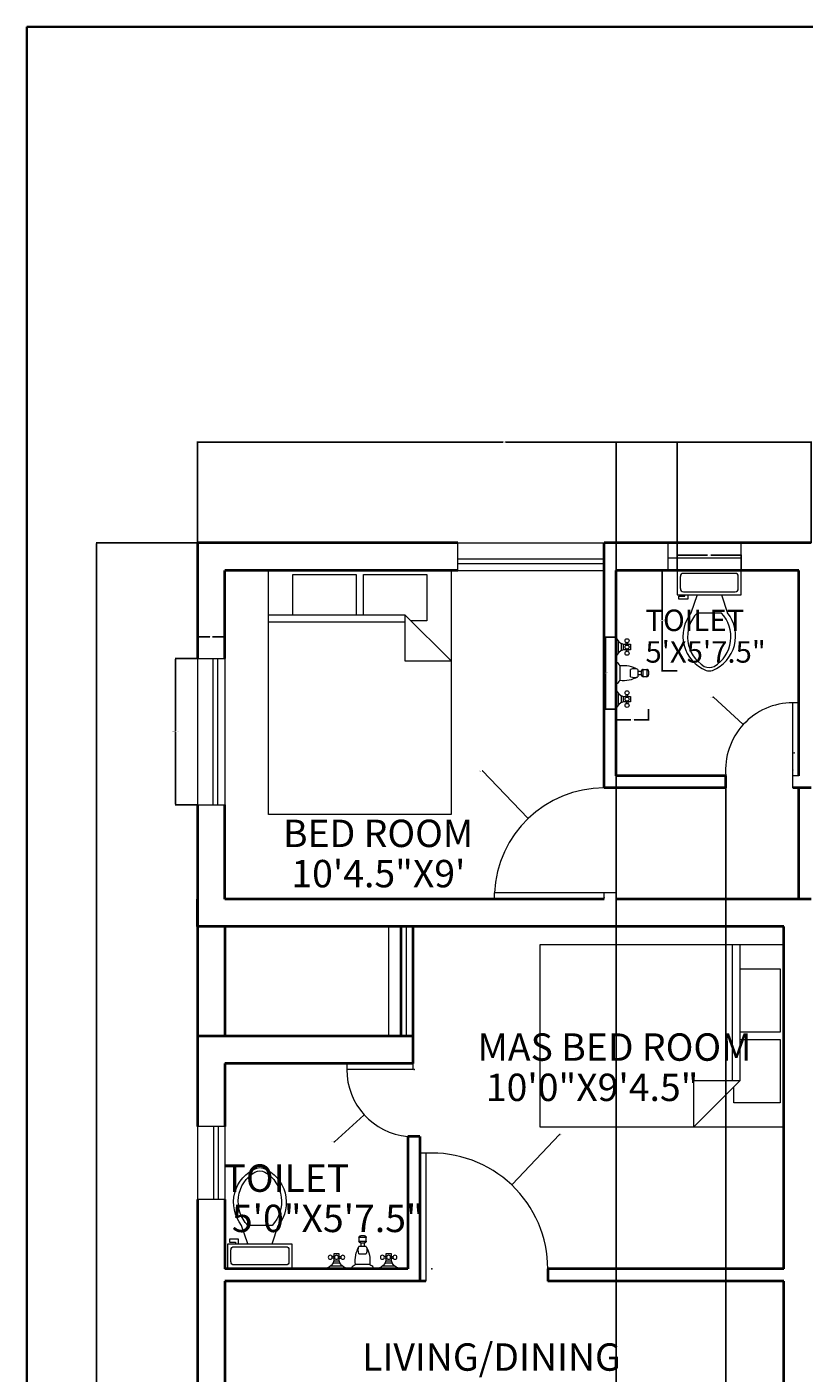
# Model space of a CAD drawing. Units: inches. Extents: x 2220 to 3422, y 783 to 1748.
# Tile 4 of 7: x 2220 to 2475, y 1306 to 1748. Entities that reach past the tile are written whole.
import ezdxf

# ---------------------------------------------------------------- set-up
doc = ezdxf.new("R2010")
doc.units = ezdxf.units.IN
for name, color, linetype, lineweight in [('A-ANNO-DIMS', 2, 'Continuous', 18), ('A-ANNO-TTLB', 7, 'Continuous', 35), ('A-AREA-IDEN', 7, 'Continuous', 18), ('A-DOOR', 3, 'Continuous', 20), ('A-FLOR-FIXT', 9, 'Continuous', 18), ('A-FURN', 8, 'Continuous', 18), ('A-GLAZ', 4, 'Continuous', 18), ('A-WALL', 7, 'Continuous', 40)]:
    doc.layers.add(name, color=color, linetype=linetype, lineweight=lineweight)
doc.styles.get("Standard").update_dxf_attribs({"font": 'arial.ttf'})
doc.dimstyles.get("Standard").update_dxf_attribs({"dimtxt": 0.18, "dimasz": 0.18, "dimexe": 0.18, "dimexo": 0.0625, "dimgap": 0.09, "dimtad": 0, "dimtih": 1, "dimtoh": 1, "dimdec": 4, "dimzin": 0, "dimdsep": 46, "dimtxsty": 'Standard', "dimcen": 0.09, "dimadec": 0, "dimazin": 0, "dimtfac": 1, "dimtdec": 4, "dimtofl": 0, "dimtmove": 0, "dimatfit": 3, "dimfxl": 1, "dimtolj": 1, "dimtzin": 0, "dimarcsym": 0})

# ---------------------------------------------------------------- blocks, each defined once
blk = doc.blocks.new('Toilet - top')
for p, q in [((9.5, -6), (9.5, -2)), ((-10, -8.5), (-8, -8.5)), ((-10, -9.5), (-10, -8.5)), ((-8, -8.5), (-8, -8)), ((-7, -8), (-7, -9.5)), ((-4, -8), (-6, -14)), ((4, -8), (6, -14)), ((-7, -9.5), (-10, -9.5)), ((4, -14), (-4, -14))]:
    blk.add_line(p, q)
blk.add_lwpolyline([(10.5, -8), (10.5, 0), (-10.5, 0), (-10.5, -8)], close=True)
for points in [[(-9.5, -2), (-9.5, -6)], [(8.5, -1), (-8.5, -1)], [(-8.5, -7), (8.5, -7)]]:
    blk.add_lwpolyline(points)
for centre, radius, start, end in [((-8.62, -1.88), 0.884, 81.8699, 188.1301), ((8.62, -1.88), 0.884, 351.8699, 98.1301), ((-8.62, -6.12), 0.884, 171.8699, 278.1301), ((8.62, -6.12), 0.884, 261.8699, 8.1301), ((3.52, -21.58), 12.17, 141.4691, 247.9714), ((4.2, -21.82), 11.33, 136.3677, 238.9468), ((-3.52, -21.58), 12.17, 292.0284, 38.5307), ((-4.2, -21.82), 11.33, 301.053, 43.6321), ((0, -27.88), 4, 245.7318, 294.2682), ((0, -29), 4, 254.8605, 285.1395)]:
    blk.add_arc(centre, radius, start, end)
blk = doc.blocks.new('Faucet - Bathroom front')
for p, q in [((-0.5, 4.25), (0.5, 4.25)), ((0.5, 3.75), (-0.5, 3.75)), ((-0.5, 3), (0.5, 3)), ((0.5, 2), (-0.5, 2)), ((-0.25, 3), (-0.25, 3.5)), ((0.25, 3.5), (0.25, 3)), ((-5, 0), (-2.25, 0)), ((-4.5087, 0.25), (-2.7408, 0.25)), ((-4, 1.625), (-4.25, 1.625)), ((-4, 1.375), (-4.25, 1.375)), ((-3.1442, 0.75), (-4.0979, 0.75)), ((-3.25, 1.625), (-3, 1.625)), ((-3.25, 1.375), (-3, 1.375)), ((-1.5, 0), (1.5, 0)), ((-1, 0.5), (1, 0.5)), ((2.25, 0), (5, 0)), ((2.7413, 0.25), (4.5092, 0.25)), ((3.25, 1.625), (3, 1.625)), ((3.25, 1.375), (3, 1.375)), ((4.1058, 0.75), (3.1521, 0.75)), ((4, 1.625), (4.25, 1.625)), ((4, 1.375), (4.25, 1.375))]:
    blk.add_line(p, q)
for points in [[(-0.5, 3.75), (-0.5, 4.25)], [(-0.25, 4.5), (0.25, 4.5)], [(0.5, 4.25), (0.5, 3.75)], [(0.25, 3.5), (-0.25, 3.5)]]:
    blk.add_lwpolyline(points)
for points in [[(-4, 1), (-4, 2), (-3.25, 2), (-3.25, 1)], [(3.25, 1), (3.25, 2), (4, 2), (4, 1)]]:
    blk.add_lwpolyline(points, close=True)
for centre in [(-4.5, 1.5), (-3.625, 1.5), (-2.75, 1.5), (2.75, 1.5), (3.625, 1.5), (4.5, 1.5)]:
    blk.add_circle(centre, 0.2795)
for centre, radius, start, end in [((-0.2575, 4.2575), 0.2426, 88.22243, 181.7776), ((-0.2575, 3.7425), 0.2426, 178.2224, 271.7776), ((0.2575, 4.2575), 0.2426, 358.2224, 91.77757), ((0.2575, 3.7425), 0.2426, 268.2224, 1.777565), ((3, 1), 4.0311, 150.2551, 187.125), ((0.6413, 2.5), 1.246, 156.3417, 203.6583), ((-3, 1), 4.0311, 352.875, 29.74488), ((-0.6413, 2.5), 1.246, 336.3417, 23.65835), ((-5.375, 1.375), 1.4252, 285.2551, 344.7449), ((-1.875, 1.375), 1.4252, 195.2551, 254.7449), ((-0.7962, -0.2038), 0.7327, 106.1502, 163.8498), ((0.7962, -0.2038), 0.7327, 16.1502, 73.84979), ((1.875, 1.375), 1.4252, 285.2551, 344.7449), ((5.375, 1.375), 1.4252, 195.2551, 254.7449)]:
    blk.add_arc(centre, radius, start, end)
blk = doc.blocks.new('Bed - Queen')
for p, q in [((0, -80.00003), (0, 0)), ((0, 0), (59.99999, 0)), ((59.99999, 0), (59.99999, -80.00003)), ((7.99999, -1.2), (28.79998, -1.2)), ((7.99999, -14.4), (7.99999, -1.2)), ((28.79998, -1.2), (28.79998, -14.4)), ((31.19999, -1.2), (51.99999, -1.2)), ((31.19999, -14.4), (31.19999, -1.2)), ((51.99999, -1.2), (51.99999, -16.4)), ((0, -14.4), (44.8, -14.4)), ((44.8, -16.8), (0, -16.8)), ((59.99999, -29.6), (44.8, -14.4)), ((44.8, -14.4), (44.8, -29.6)), ((51.99999, -16.4), (46.79936, -16.4)), ((44.8, -29.6), (59.99999, -29.6)), ((59.99999, -80.00003), (0, -80.00003))]:
    blk.add_line(p, q)
blk = doc.blocks.new('WIN-48-OFFSET-B')
for p, q in [((0, 48), (9, 48)), ((0, 48), (0, 0)), ((5, 48), (5, 0)), ((6.5, 48), (6.5, 0)), ((9, 48), (9, 0)), ((0, 0), (9, 0))]:
    blk.add_line(p, q)
blk = doc.blocks.new('*D21')
at = {"layer": 'A-ANNO-DIMS', "color": 0, "lineweight": -2, "transparency": 16777216}
for p, q in [((2433.53, 1569.38), (2428.45, 1569.38)), ((2428.63, 1569.2), (2428.63, 1553.04)), ((2428.63, 1536.51), (2428.63, 1552.67)), ((2433.53, 1536.33), (2428.45, 1536.33))]:
    blk.add_line(p, q, dxfattribs=at)
at = {"layer": 'A-ANNO-DIMS', "color": 0, "transparency": 16777216}
for points in [[(2428.6, 1569.2), (2428.66, 1569.2), (2428.63, 1569.38)], [(2428.6, 1536.51), (2428.66, 1536.51), (2428.63, 1536.33)]]:
    blk.add_solid(points, dxfattribs=at)
at = {"layer": 'Defpoints', "color": 0, "transparency": 16777216}
for p in [(2428.63, 1569.38), (2433.59, 1569.38), (2433.59, 1536.33)]:
    blk.add_point(p, dxfattribs=at)
at = {"layer": 'A-ANNO-DIMS', "color": 0, "transparency": 16777216, "insert": (2428.63, 1552.86), "char_height": 0.18, "attachment_point": 5}
blk.add_mtext('\\A1;WC 33 TYP.', dxfattribs=at)
blk = doc.blocks.new('*D22')
at = {"layer": 'A-ANNO-DIMS', "color": 0, "lineweight": -2, "transparency": 16777216}
for p, q in [((2433.59, 1569.44), (2433.59, 1574.52)), ((2433.77, 1574.34), (2443.56, 1574.34)), ((2454.41, 1574.34), (2444.62, 1574.34)), ((2454.59, 1569.44), (2454.59, 1574.52))]:
    blk.add_line(p, q, dxfattribs=at)
at = {"layer": 'A-ANNO-DIMS', "color": 0, "transparency": 16777216}
for points in [[(2433.77, 1574.37), (2433.77, 1574.31), (2433.59, 1574.34)], [(2454.41, 1574.37), (2454.41, 1574.31), (2454.59, 1574.34)]]:
    blk.add_solid(points, dxfattribs=at)
at = {"layer": 'Defpoints', "color": 0, "transparency": 16777216}
for p in [(2454.59, 1574.34), (2433.59, 1569.38), (2454.59, 1569.38)]:
    blk.add_point(p, dxfattribs=at)
at = {"layer": 'A-ANNO-DIMS', "color": 0, "transparency": 16777216, "insert": (2444.09, 1574.34), "char_height": 0.18, "attachment_point": 5}
blk.add_mtext('\\A1;21 TYP.', dxfattribs=at)
blk = doc.blocks.new('*D23')
at = {"layer": 'A-ANNO-DIMS', "color": 0, "lineweight": -2, "transparency": 16777216}
for p, q in [((2413.48, 1547.45), (2409.82, 1547.45)), ((2410, 1547.27), (2410, 1535.82)), ((2410, 1524.01), (2410, 1535.46)), ((2413.48, 1523.83), (2409.82, 1523.83))]:
    blk.add_line(p, q, dxfattribs=at)
at = {"layer": 'A-ANNO-DIMS', "color": 0, "transparency": 16777216}
for points in [[(2409.97, 1547.27), (2410.03, 1547.27), (2410, 1547.45)], [(2409.97, 1524.01), (2410.03, 1524.01), (2410, 1523.83)]]:
    blk.add_solid(points, dxfattribs=at)
at = {"layer": 'Defpoints', "color": 0, "transparency": 16777216}
for p in [(2413.55, 1547.45), (2410, 1523.83), (2413.55, 1523.83)]:
    blk.add_point(p, dxfattribs=at)
at = {"layer": 'A-ANNO-DIMS', "color": 0, "transparency": 16777216, "insert": (2410, 1535.64), "char_height": 0.18, "attachment_point": 5}
blk.add_mtext('\\A1;LAV. TAP 24 TYP.', dxfattribs=at)
blk = doc.blocks.new('*D24')
at = {"layer": 'A-ANNO-DIMS', "color": 0, "lineweight": -2, "transparency": 16777216}
for p, q in [((2413.55, 1523.77), (2413.55, 1520.11)), ((2424.18, 1523.77), (2424.18, 1520.11)), ((2413.73, 1520.29), (2418.34, 1520.29)), ((2424, 1520.29), (2419.38, 1520.29))]:
    blk.add_line(p, q, dxfattribs=at)
at = {"layer": 'A-ANNO-DIMS', "color": 0, "transparency": 16777216}
for points in [[(2413.73, 1520.32), (2413.73, 1520.26), (2413.55, 1520.29)], [(2424, 1520.32), (2424, 1520.26), (2424.18, 1520.29)]]:
    blk.add_solid(points, dxfattribs=at)
at = {"layer": 'Defpoints', "color": 0, "transparency": 16777216}
for p in [(2413.55, 1523.83), (2424.18, 1523.83), (2424.18, 1520.29)]:
    blk.add_point(p, dxfattribs=at)
at = {"layer": 'A-ANNO-DIMS', "color": 0, "transparency": 16777216, "insert": (2418.86, 1520.29), "char_height": 0.18, "attachment_point": 5}
blk.add_mtext('\\A1;11 TYP.', dxfattribs=at)
blk = doc.blocks.new('*D49')
at = {"layer": 'A-ANNO-DIMS', "color": 0, "lineweight": -2, "transparency": 16777216}
for p, q in [((2275.98, 1540.39), (2268.67, 1540.39)), ((2268.85, 1540.21), (2268.85, 1516.57)), ((2268.85, 1492.57), (2268.85, 1516.21)), ((2275.98, 1492.39), (2268.67, 1492.39))]:
    blk.add_line(p, q, dxfattribs=at)
at = {"layer": 'A-ANNO-DIMS', "color": 0, "transparency": 16777216}
for points in [[(2268.82, 1540.21), (2268.88, 1540.21), (2268.85, 1540.39)], [(2268.82, 1492.57), (2268.88, 1492.57), (2268.85, 1492.39)]]:
    blk.add_solid(points, dxfattribs=at)
at = {"layer": 'Defpoints', "color": 0, "transparency": 16777216}
for p in [(2268.85, 1540.39), (2276.05, 1540.39), (2276.05, 1492.39)]:
    blk.add_point(p, dxfattribs=at)
at = {"layer": 'A-ANNO-DIMS', "color": 0, "transparency": 16777216, "insert": (2268.85, 1516.39), "char_height": 0.18, "attachment_point": 5}
blk.add_mtext('\\A1;WINDOW B 48 TYP.', dxfattribs=at)
blk = doc.blocks.new('*D50')
at = {"layer": 'A-ANNO-DIMS', "color": 0, "lineweight": -2, "transparency": 16777216}
for p, q in [((2276.05, 1540.45), (2276.05, 1547.77)), ((2276.23, 1547.59), (2280.09, 1547.59)), ((2284.87, 1547.59), (2281, 1547.59)), ((2285.05, 1540.45), (2285.05, 1547.77))]:
    blk.add_line(p, q, dxfattribs=at)
at = {"layer": 'A-ANNO-DIMS', "color": 0, "transparency": 16777216}
for points in [[(2276.23, 1547.62), (2276.23, 1547.56), (2276.05, 1547.59)], [(2284.87, 1547.62), (2284.87, 1547.56), (2285.05, 1547.59)]]:
    blk.add_solid(points, dxfattribs=at)
at = {"layer": 'Defpoints', "color": 0, "transparency": 16777216}
for p in [(2285.05, 1547.59), (2276.05, 1540.39), (2285.05, 1540.39)]:
    blk.add_point(p, dxfattribs=at)
at = {"layer": 'A-ANNO-DIMS', "color": 0, "transparency": 16777216, "insert": (2280.55, 1547.59), "char_height": 0.18, "attachment_point": 5}
blk.add_mtext('\\A1;9 TYP.', dxfattribs=at)
blk = doc.blocks.new('*D54')
at = {"layer": 'A-ANNO-DIMS', "color": 0, "lineweight": -2, "transparency": 16777216}
for p, q in [((2275.98, 1578.39), (2242.72, 1578.39)), ((2242.9, 1578.21), (2242.9, 1255.07)), ((2242.9, 931.57), (2242.9, 1254.71)), ((2275.98, 931.39), (2242.72, 931.39))]:
    blk.add_line(p, q, dxfattribs=at)
at = {"layer": 'A-ANNO-DIMS', "color": 0, "transparency": 16777216}
for points in [[(2242.87, 1578.21), (2242.93, 1578.21), (2242.9, 1578.39)], [(2242.87, 931.57), (2242.93, 931.57), (2242.9, 931.39)]]:
    blk.add_solid(points, dxfattribs=at)
at = {"layer": 'Defpoints', "color": 0, "transparency": 16777216}
for p in [(2242.9, 1578.39), (2276.05, 1578.39), (2276.05, 931.39)]:
    blk.add_point(p, dxfattribs=at)
at = {"layer": 'A-ANNO-DIMS', "color": 0, "transparency": 16777216, "insert": (2242.9, 1254.89), "char_height": 0.18, "attachment_point": 5}
blk.add_mtext('\\A1;647', dxfattribs=at)
blk = doc.blocks.new('*D58')
at = {"layer": 'A-ANNO-DIMS', "color": 0, "lineweight": -2, "transparency": 16777216}
for p, q in [((2276.05, 1578.45), (2276.05, 1611.72)), ((2276.23, 1611.54), (2376.4, 1611.54)), ((2477.37, 1611.54), (2377.19, 1611.54)), ((2477.55, 1578.45), (2477.55, 1611.72))]:
    blk.add_line(p, q, dxfattribs=at)
at = {"layer": 'A-ANNO-DIMS', "color": 0, "transparency": 16777216}
for points in [[(2276.23, 1611.57), (2276.23, 1611.51), (2276.05, 1611.54)], [(2477.37, 1611.57), (2477.37, 1611.51), (2477.55, 1611.54)]]:
    blk.add_solid(points, dxfattribs=at)
at = {"layer": 'Defpoints', "color": 0, "transparency": 16777216}
for p in [(2477.55, 1611.54), (2276.05, 1578.39), (2477.55, 1578.39)]:
    blk.add_point(p, dxfattribs=at)
at = {"layer": 'A-ANNO-DIMS', "color": 0, "transparency": 16777216, "insert": (2376.8, 1611.54), "char_height": 0.18, "attachment_point": 5}
blk.add_mtext('\\A1;201.5', dxfattribs=at)
blk = doc.blocks.new('*D72')
at = {"layer": 'A-ANNO-DIMS', "color": 0, "lineweight": -2, "transparency": 16777216}
for p, q in [((2413.55, 1569.45), (2413.55, 1611.72)), ((2413.73, 1611.54), (2423.1, 1611.54)), ((2433.41, 1611.54), (2424.04, 1611.54)), ((2433.59, 1569.44), (2433.59, 1611.72))]:
    blk.add_line(p, q, dxfattribs=at)
at = {"layer": 'A-ANNO-DIMS', "color": 0, "transparency": 16777216}
for points in [[(2413.73, 1611.57), (2413.73, 1611.51), (2413.55, 1611.54)], [(2433.41, 1611.57), (2433.41, 1611.51), (2433.59, 1611.54)]]:
    blk.add_solid(points, dxfattribs=at)
at = {"layer": 'Defpoints', "color": 0, "transparency": 16777216}
for p in [(2433.59, 1611.54), (2413.55, 1569.39), (2433.59, 1569.38)]:
    blk.add_point(p, dxfattribs=at)
at = {"layer": 'A-ANNO-DIMS', "color": 0, "transparency": 16777216, "insert": (2423.57, 1611.54), "char_height": 0.18, "attachment_point": 5}
blk.add_mtext('\\A1;20.045', dxfattribs=at)
blk = doc.blocks.new('*D73')
at = {"layer": 'A-ANNO-DIMS', "color": 0, "lineweight": -2, "transparency": 16777216}
for p, q in [((2413.55, 1501.83), (2413.55, 898.06)), ((2449.55, 1501.83), (2449.55, 898.06)), ((2413.73, 898.24), (2431.33, 898.24)), ((2449.37, 898.24), (2431.77, 898.24))]:
    blk.add_line(p, q, dxfattribs=at)
at = {"layer": 'A-ANNO-DIMS', "color": 0, "transparency": 16777216}
for points in [[(2413.73, 898.27), (2413.73, 898.21), (2413.55, 898.24)], [(2449.37, 898.27), (2449.37, 898.21), (2449.55, 898.24)]]:
    blk.add_solid(points, dxfattribs=at)
at = {"layer": 'Defpoints', "color": 0, "transparency": 16777216}
for p in [(2413.55, 1501.89), (2449.55, 1501.89), (2449.55, 898.24)]:
    blk.add_point(p, dxfattribs=at)
at = {"layer": 'A-ANNO-DIMS', "color": 0, "transparency": 16777216, "insert": (2431.55, 898.24), "char_height": 0.18, "attachment_point": 5}
blk.add_mtext('\\A1;36', dxfattribs=at)
blk = doc.blocks.new('*D78')
at = {"layer": 'A-ANNO-DIMS', "color": 0, "lineweight": -2, "transparency": 16777216}
for p, q in [((2394.93, 1384.03), (2379.33, 1367.61)), ((2395.11, 1384.03), (2394.93, 1384.03)), ((2352.91, 1339.89), (2353.09, 1339.89)), ((2353, 1339.8), (2353, 1339.98))]:
    blk.add_line(p, q, dxfattribs=at)
at = {"layer": 'A-ANNO-DIMS', "color": 0, "transparency": 16777216}
blk.add_solid([(2379.31, 1367.63), (2379.35, 1367.59), (2379.2, 1367.48)], dxfattribs=at)
at = {"layer": 'Defpoints', "color": 0, "transparency": 16777216}
for p in [(2379.2, 1367.48), (2353, 1339.89)]:
    blk.add_point(p, dxfattribs=at)
at = {"layer": 'A-ANNO-DIMS', "color": 0, "transparency": 16777216, "insert": (2395.59, 1384.03), "char_height": 0.18, "attachment_point": 5}
blk.add_mtext('\\A1;R38.05', dxfattribs=at)
blk = doc.blocks.new('*D79')
at = {"layer": 'A-ANNO-DIMS', "color": 0, "lineweight": -2, "transparency": 16777216}
for p, q in [((2369.48, 1503.48), (2369.66, 1503.48)), ((2369.66, 1503.48), (2384.49, 1488)), ((2409.46, 1461.86), (2409.64, 1461.86)), ((2409.55, 1461.77), (2409.55, 1461.95))]:
    blk.add_line(p, q, dxfattribs=at)
at = {"layer": 'A-ANNO-DIMS', "color": 0, "transparency": 16777216}
blk.add_solid([(2384.51, 1488.02), (2384.47, 1487.98), (2384.62, 1487.87)], dxfattribs=at)
at = {"layer": 'Defpoints', "color": 0, "transparency": 16777216}
for p in [(2384.62, 1487.87), (2409.55, 1461.86)]:
    blk.add_point(p, dxfattribs=at)
at = {"layer": 'A-ANNO-DIMS', "color": 0, "transparency": 16777216, "insert": (2369, 1503.48), "char_height": 0.18, "attachment_point": 5}
blk.add_mtext('\\A1;R36.03', dxfattribs=at)
blk = doc.blocks.new('*D82')
at = {"layer": 'A-ANNO-DIMS', "color": 0, "lineweight": -2, "transparency": 16777216}
for p, q in [((2511.68, 1535.13), (2496.94, 1525.58)), ((2511.86, 1535.13), (2511.68, 1535.13)), ((2471.88, 1509.39), (2472.06, 1509.39)), ((2471.97, 1509.3), (2471.97, 1509.48))]:
    blk.add_line(p, q, dxfattribs=at)
at = {"layer": 'A-ANNO-DIMS', "color": 0, "transparency": 16777216}
blk.add_solid([(2496.92, 1525.6), (2496.96, 1525.55), (2496.79, 1525.48)], dxfattribs=at)
at = {"layer": 'Defpoints', "color": 0, "transparency": 16777216}
for p in [(2496.79, 1525.48), (2471.97, 1509.39)]:
    blk.add_point(p, dxfattribs=at)
at = {"layer": 'A-ANNO-DIMS', "color": 0, "transparency": 16777216, "insert": (2512.54, 1535.13), "char_height": 0.18, "attachment_point": 5}
blk.add_mtext('\\A1;2X R29.58', dxfattribs=at)
blk = doc.blocks.new('*D85')
at = {"layer": 'A-ANNO-DIMS', "color": 0, "lineweight": -2, "transparency": 16777216}
for p, q in [((2347.06, 1405.39), (2347.24, 1405.39)), ((2347.15, 1405.3), (2347.15, 1405.48)), ((2320.98, 1381.61), (2330.66, 1390.4)), ((2320.8, 1381.61), (2320.98, 1381.61))]:
    blk.add_line(p, q, dxfattribs=at)
at = {"layer": 'A-ANNO-DIMS', "color": 0, "transparency": 16777216}
blk.add_solid([(2330.64, 1390.43), (2330.68, 1390.38), (2330.79, 1390.52)], dxfattribs=at)
at = {"layer": 'Defpoints', "color": 0, "transparency": 16777216}
for p in [(2347.15, 1405.39), (2330.79, 1390.52)]:
    blk.add_point(p, dxfattribs=at)
at = {"layer": 'A-ANNO-DIMS', "color": 0, "transparency": 16777216, "insert": (2320.41, 1381.61), "char_height": 0.18, "attachment_point": 5}
blk.add_mtext('\\A1;R22.1', dxfattribs=at)
blk = doc.blocks.new('*D86')
at = {"layer": 'A-ANNO-DIMS', "color": 0, "lineweight": -2, "transparency": 16777216}
for p, q in [((2445.32, 1527.68), (2445.5, 1527.68)), ((2445.5, 1527.68), (2455.14, 1518.85)), ((2471.55, 1503.72), (2471.55, 1503.9)), ((2471.46, 1503.81), (2471.64, 1503.81))]:
    blk.add_line(p, q, dxfattribs=at)
at = {"layer": 'A-ANNO-DIMS', "color": 0, "transparency": 16777216}
blk.add_solid([(2455.16, 1518.87), (2455.12, 1518.83), (2455.27, 1518.73)], dxfattribs=at)
at = {"layer": 'Defpoints', "color": 0, "transparency": 16777216}
for p in [(2455.27, 1518.73), (2471.55, 1503.81)]:
    blk.add_point(p, dxfattribs=at)
at = {"layer": 'A-ANNO-DIMS', "color": 0, "transparency": 16777216, "insert": (2444.77, 1527.68), "char_height": 0.18, "attachment_point": 5}
blk.add_mtext('\\A1;R22.083', dxfattribs=at)

msp = doc.modelspace()

# ---------------------------------------------------------------- linework, layer by layer
at = {"layer": 'A-ANNO-TTLB'}
msp.add_lwpolyline([(2220.0037, 1747.9465), (3422.343, 1747.9465), (3422.343, 782.804), (2220.0037, 782.804)], close=True, dxfattribs=at)
at = {"layer": 'A-DOOR'}
for p, q in [((2471.5466, 1497.8907), (2471.5466, 1525.8907)), ((2473.5466, 1525.8907), (2471.5466, 1525.8907)), ((2473.5466, 1501.8907), (2471.5466, 1501.8907)), ((2373.5466, 1461.3907), (2373.5466, 1463.3907)), ((2413.5466, 1463.3907), (2373.5466, 1463.3907)), ((2409.5466, 1461.3907), (2409.5466, 1463.3907)), ((2413.5466, 1461.3907), (2413.5466, 1463.3907)), ((2325.0466, 1407.3907), (2325.0466, 1405.3907)), ((2346.7966, 1407.3907), (2346.7966, 1405.3907)), ((2346.7966, 1405.3907), (2325.0466, 1405.3907)), ((2351.0466, 1377.8907), (2349.0466, 1377.8907)), ((2351.0466, 1377.8907), (2351.0466, 1335.8907))]:
    msp.add_line(p, q, dxfattribs=at)
for centre, radius, start, end in [((2471.5466, 1503.8074), 22.0833, 90, 184.979106), ((2409.5466, 1461.8581), 36.0326, 90, 177.56225), ((2347.1466, 1405.3907), 22.1, 180, 264.547378), ((2352.9966, 1339.8907), 38.05, 0, 92.937601)]:
    msp.add_arc(centre, radius, start, end, dxfattribs=at)
at = {"layer": 'A-GLAZ'}
for p, q in [((2361.5466, 1569.3907), (2361.5466, 1578.3907)), ((2361.5466, 1578.3907), (2409.5466, 1578.3907)), ((2430.5466, 1569.3907), (2430.5466, 1578.3907)), ((2454.5466, 1569.3907), (2454.5466, 1578.3907)), ((2361.5466, 1573.1407), (2409.5466, 1573.1407)), ((2361.5466, 1571.6407), (2409.5466, 1571.6407)), ((2454.5466, 1573.3907), (2430.5466, 1573.3907)), ((2454.5466, 1573.3907), (2430.5466, 1573.3907)), ((2361.5466, 1569.3907), (2409.5466, 1569.3907)), ((2338.7966, 1452.3907), (2338.7966, 1416.3907)), ((2344.5466, 1452.3907), (2344.5466, 1416.3907)), ((2285.0466, 1386.6407), (2276.0466, 1386.6407)), ((2276.0466, 1386.6407), (2276.0466, 1362.6407)), ((2281.2966, 1386.6407), (2281.2966, 1362.6407)), ((2282.7966, 1386.6407), (2282.7966, 1362.6407)), ((2285.0466, 1386.6407), (2285.0466, 1362.6407)), ((2285.0466, 1362.6407), (2276.0466, 1362.6407))]:
    msp.add_line(p, q, dxfattribs=at)
at = {"layer": 'A-WALL'}
for p, q in [((2276.0466, 1578.3907), (2276.0466, 1540.3907)), ((2361.5466, 1578.3907), (2276.0466, 1578.3907)), ((2477.5466, 1578.3907), (2409.5466, 1578.3907)), ((2409.5466, 1497.8907), (2409.5466, 1578.3907)), ((2361.5466, 1569.3907), (2285.0466, 1569.3907)), ((2285.0466, 1540.3907), (2285.0466, 1569.3907)), ((2473.5466, 1569.3907), (2413.5466, 1569.3907)), ((2413.5466, 1501.8907), (2413.5466, 1569.3907)), ((2473.5466, 1569.3907), (2413.5466, 1569.3907)), ((2473.5466, 1501.8907), (2473.5466, 1569.3907)), ((2449.5466, 1501.8907), (2413.5466, 1501.8907)), ((2449.5466, 1497.8907), (2449.5466, 1501.8907)), ((2449.5466, 1497.8907), (2409.5466, 1497.8907)), ((2477.5466, 1497.8907), (2471.5466, 1497.8907)), ((2473.5466, 1461.3907), (2473.5466, 1497.8907)), ((2276.0466, 1492.3907), (2276.0466, 1452.3907)), ((2285.0466, 1461.3907), (2285.0466, 1492.3907)), ((2276.0466, 1452.3907), (2276.0466, 1461.3907)), ((2409.5466, 1461.3907), (2285.0466, 1461.3907)), ((2477.5466, 1461.3907), (2413.5466, 1461.3907)), ((2468.5466, 1452.3907), (2276.0466, 1452.3907)), ((2276.0466, 1452.3907), (2276.0466, 1416.3907)), ((2285.0466, 1452.3907), (2285.0466, 1416.3907)), ((2342.7966, 1452.3907), (2342.7966, 1416.3907)), ((2346.7966, 1452.3907), (2346.7966, 1416.3907)), ((2468.5466, 1339.8907), (2468.5466, 1452.3907)), ((2276.0466, 1416.3907), (2276.0466, 1386.6407)), ((2346.7966, 1416.3907), (2276.0466, 1416.3907)), ((2346.7966, 1416.3907), (2346.7966, 1407.3907)), ((2285.0466, 1407.3907), (2285.0466, 1386.6407)), ((2346.7966, 1407.3907), (2285.0466, 1407.3907)), ((2349.0466, 1383.3907), (2345.0466, 1383.3907)), ((2345.0466, 1383.3907), (2345.0466, 1339.8907)), ((2349.0466, 1383.3907), (2349.0466, 1335.8907)), ((2276.0466, 1362.6407), (2276.0466, 1211.8907)), ((2285.0466, 1362.6407), (2285.0466, 1339.8907)), ((2345.0466, 1339.8907), (2285.0466, 1339.8907)), ((2285.0466, 1335.8907), (2285.0466, 1227.8907)), ((2351.0466, 1335.8907), (2285.0466, 1335.8907)), ((2468.5466, 1339.8907), (2391.0466, 1339.8907)), ((2391.0466, 1339.8907), (2391.0466, 1335.8907)), ((2468.5466, 1335.8907), (2391.0466, 1335.8907)), ((2468.5466, 1271.8907), (2468.5466, 1335.8907))]:
    msp.add_line(p, q, dxfattribs=at)

# ---------------------------------------------------------------- block references
at = {"layer": 'A-FLOR-FIXT'}
msp.add_blockref('Toilet - top', (2444.0919, 1569.3782), dxfattribs=at)
at = {"layer": 'A-FLOR-FIXT', "yscale": 2.361580970438625, "zscale": 2.361580970438625}
for p, xscale, rotation in [((2413.5466, 1535.6407), 2.361580970438625, 270), ((2330.2379, 1340.1349), -2.361580970438625, 359.9999999999942)]:
    msp.add_blockref('Faucet - Bathroom front', p, dxfattribs=dict(at, xscale=xscale, rotation=rotation))
at = {"layer": 'A-FLOR-FIXT', "xscale": -1, "rotation": 180}
msp.add_blockref('Toilet - top', (2296.5234, 1340.1591), dxfattribs=at)
at = {"layer": 'A-FURN'}
msp.add_blockref('Bed - Queen', (2299.3508, 1569.22), dxfattribs=at)
at = {"layer": 'A-FURN', "rotation": 270}
msp.add_blockref('Bed - Queen', (2468.5466, 1446.4671), dxfattribs=at)
at = {"layer": 'A-GLAZ'}
msp.add_blockref('WIN-48-OFFSET-B', (2276.047, 1492.391), dxfattribs=at)

# ---------------------------------------------------------------- texts
at = {"layer": 'A-AREA-IDEN'}
for s, height, p in [('  TOILET', 7.06044, (2418.8302, 1549.44)), ('  5\'X5\'7.5"', 7.060438, (2418.8302, 1539.0634)), ('BED ROOM', 9, (2304.104, 1478.4746)), (' 10\'4.5"X9\'', 9, (2304.104, 1465.2475)), ('MAS BED ROOM', 9, (2367.9804, 1408.2556)), (' 10\'0"X9\'4.5"', 9, (2367.9804, 1395.0286)), ('TOILET', 9, (2284.5626, 1365.1913)), (' 5\'0"X5\'7.5"', 9, (2284.5626, 1351.9643)), ('LIVING/DINING', 9, (2330.095, 1306.4078))]:
    msp.add_text(s, height=height, dxfattribs=at).set_placement(p)

# ---------------------------------------------------------------- dimensions: what is measured, and where the dimension line sits
at = {"layer": 'A-ANNO-DIMS'}
for base, p1, p2, override, picture, middle in [((2477.5466, 1611.5407), (2276.0466, 1578.3907), (2477.5466, 1578.3907), {"dimdec": 1, "dimlfac": 1, "dimrnd": 0, "dimzin": 0, "dimdsep": 46, "dimlunit": 2}, '*D58', (2376.7966, 1611.5407)), ((2433.5919, 1611.5407), (2413.5466, 1569.3907), (2433.5919, 1569.3782), {"dimdec": 3, "dimlfac": 1, "dimrnd": 0, "dimzin": 0, "dimdsep": 46, "dimlunit": 2}, '*D72', (2423.5692, 1611.5407)), ((2449.5466, 898.2407), (2413.5466, 1501.8907), (2449.5466, 1501.8907), {"dimdec": 0, "dimlfac": 1, "dimrnd": 0, "dimzin": 0, "dimdsep": 46, "dimlunit": 2}, '*D73', (2431.5466, 898.2407))]:
    dim = msp.add_linear_dim(base=base, p1=p1, p2=p2, dimstyle='Standard', override=override, dxfattribs=at)
    dim.commit()
    dim.dimension.update_dxf_attribs({"geometry": picture, "text_midpoint": middle})
dim = msp.add_linear_dim(base=(2242.8966, 1578.3907), p1=(2276.0466, 931.3907), p2=(2276.0466, 1578.3907), angle=90, dimstyle='Standard', override={"dimdec": 0, "dimlfac": 1, "dimrnd": 0, "dimzin": 0, "dimdsep": 46, "dimlunit": 2}, dxfattribs=at)
dim.commit()
dim.dimension.update_dxf_attribs({"geometry": '*D54', "text_midpoint": (2242.8966, 1254.8907)})
for base, p1, p2, picture, middle in [((2454.5919, 1574.3352), (2433.5919, 1569.3782), (2454.5919, 1569.3782), '*D22', (2444.0919, 1574.3352)), ((2285.0466, 1547.5907), (2276.0466, 1540.3907), (2285.0466, 1540.3907), '*D50', (2280.5466, 1547.5907)), ((2424.1786, 1520.2904), (2413.5466, 1523.8328), (2424.1786, 1523.8328), '*D24', (2418.8626, 1520.2904))]:
    dim = msp.add_linear_dim(base=base, p1=p1, p2=p2, text='<> TYP.', dimstyle='Standard', override={"dimdec": 0, "dimlfac": 1, "dimrnd": 0, "dimzin": 0, "dimdsep": 46, "dimlunit": 2}, dxfattribs=at)
    dim.commit()
    dim.dimension.update_dxf_attribs({"geometry": picture, "text_midpoint": middle})
for base, p1, p2, angle, text, picture, middle in [((2428.6349, 1569.3782), (2433.5919, 1536.332), (2433.5919, 1569.3782), 90, 'WC <> TYP.', '*D21', (2428.6349, 1552.8551)), ((2410.0043, 1523.8328), (2413.5466, 1547.4486), (2413.5466, 1523.8328), 270, 'LAV. TAP <> TYP.', '*D23', (2410.0043, 1535.6407)), ((2268.8466, 1540.3907), (2276.0466, 1492.3907), (2276.0466, 1540.3907), 90, 'WINDOW B <> TYP.', '*D49', (2268.8466, 1516.3907))]:
    dim = msp.add_linear_dim(base=base, p1=p1, p2=p2, angle=angle, text=text, dimstyle='Standard', override={"dimdec": 0, "dimlfac": 1, "dimrnd": 0, "dimzin": 0, "dimdsep": 46, "dimlunit": 2}, dxfattribs=at)
    dim.commit()
    dim.dimension.update_dxf_attribs({"geometry": picture, "text_midpoint": middle})
dim = msp.add_radius_dim(center=(2471.9681, 1509.3907), mpoint=(2496.7892, 1525.4781), text='2X <>', dimstyle='Standard', override={"dimdec": 2, "dimlfac": 1, "dimrnd": 0, "dimzin": 0, "dimdsep": 46, "dimlunit": 2}, dxfattribs=at)
dim.commit()
dim.dimension.update_dxf_attribs({"geometry": '*D82', "text_midpoint": (2512.5368, 1535.1306), "dimtype": 164})
for center, mpoint, override, picture, middle in [((2471.5466, 1503.8074), (2455.2681, 1518.7299), {"dimdec": 3, "dimlfac": 1, "dimrnd": 0, "dimzin": 0, "dimdsep": 46, "dimlunit": 2}, '*D86', (2444.7712, 1527.6834)), ((2409.5466, 1461.8581), (2384.6151, 1487.8729), {"dimdec": 2, "dimlfac": 1, "dimrnd": 0, "dimzin": 0, "dimdsep": 46, "dimlunit": 2}, '*D79', (2368.9964, 1503.4817)), ((2347.1466, 1405.3907), (2330.7938, 1390.5248), {"dimdec": 1, "dimlfac": 1, "dimrnd": 0, "dimzin": 0, "dimdsep": 46, "dimlunit": 2}, '*D85', (2320.4095, 1381.6053)), ((2352.9966, 1339.8907), (2379.2037, 1367.4767), {"dimdec": 2, "dimlfac": 1, "dimrnd": 0, "dimzin": 0, "dimdsep": 46, "dimlunit": 2}, '*D78', (2395.5885, 1384.0284))]:
    dim = msp.add_radius_dim(center=center, mpoint=mpoint, dimstyle='Standard', override=override, dxfattribs=at)
    dim.commit()
    dim.dimension.update_dxf_attribs({"geometry": picture, "text_midpoint": middle, "dimtype": 164})

doc.saveas('drawing.dxf')
